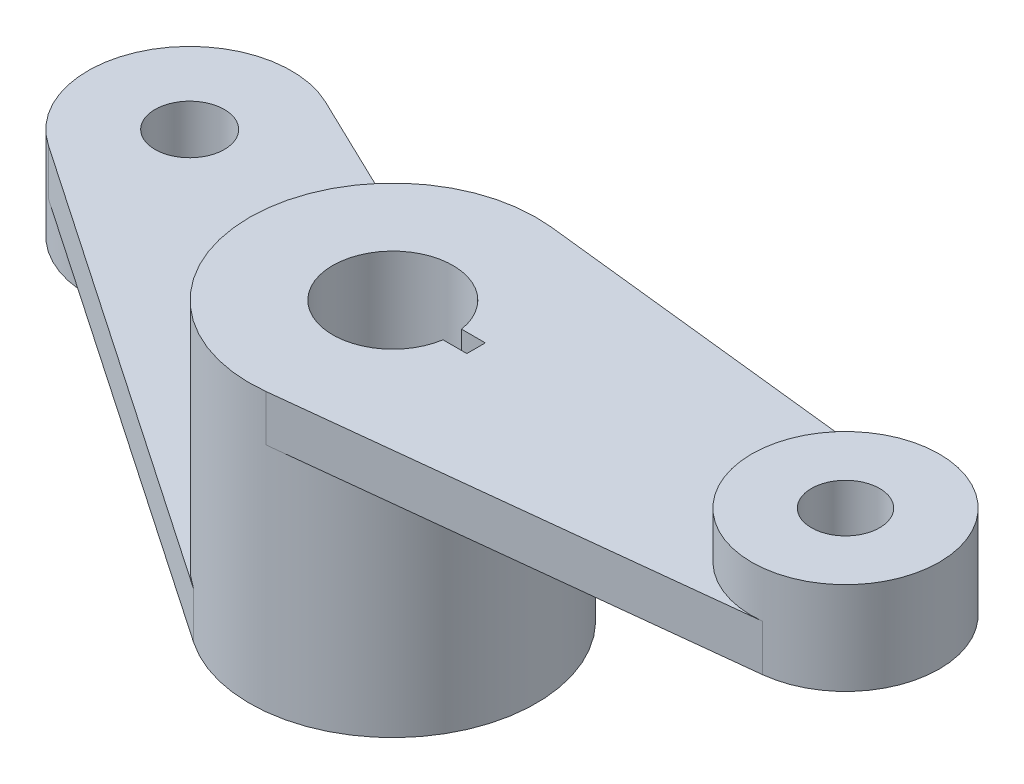
ISO-10303-21;
HEADER;
FILE_DESCRIPTION(('STEP AP214'),'2;1');
FILE_NAME('part.step','',(''),(''),'','','');
FILE_SCHEMA(('AUTOMOTIVE_DESIGN { 1 0 10303 214 1 1 1 1 }'));
ENDSEC;
DATA;
#1=APPLICATION_CONTEXT('core data for automotive mechanical design processes');
#2=APPLICATION_PROTOCOL_DEFINITION('international standard','automotive_design',2000,#1);
#3=PRODUCT_CONTEXT('',#1,'mechanical');
#4=PRODUCT('Part','Part','',(#3));
#5=PRODUCT_RELATED_PRODUCT_CATEGORY('part','',(#4));
#6=PRODUCT_DEFINITION_FORMATION('','',#4);
#7=PRODUCT_DEFINITION_CONTEXT('part definition',#1,'design');
#8=PRODUCT_DEFINITION('design','',#6,#7);
#9=PRODUCT_DEFINITION_SHAPE('','',#8);
#10=(LENGTH_UNIT() NAMED_UNIT(*) SI_UNIT(.MILLI.,.METRE.));
#11=(NAMED_UNIT(*) PLANE_ANGLE_UNIT() SI_UNIT($,.RADIAN.));
#12=(NAMED_UNIT(*) SI_UNIT($,.STERADIAN.) SOLID_ANGLE_UNIT());
#13=UNCERTAINTY_MEASURE_WITH_UNIT(LENGTH_MEASURE(1.E-05),#10,'distance_accuracy_value','');
#14=(GEOMETRIC_REPRESENTATION_CONTEXT(3) GLOBAL_UNCERTAINTY_ASSIGNED_CONTEXT((#13)) GLOBAL_UNIT_ASSIGNED_CONTEXT((#10,
#11,#12)) REPRESENTATION_CONTEXT('',''));
#15=CARTESIAN_POINT('',(0.,0.,0.));
#16=DIRECTION('',(0.,0.,1.));
#17=DIRECTION('',(1.,0.,0.));
#18=AXIS2_PLACEMENT_3D('',#15,#16,#17);
#19=CARTESIAN_POINT('',(0.,0.,0.));
#20=DIRECTION('',(0.,1.,0.));
#21=DIRECTION('',(0.,0.,1.));
#22=AXIS2_PLACEMENT_3D('',#19,#20,#21);
#23=PLANE('',#22);
#24=CARTESIAN_POINT('',(0.,0.,0.));
#25=DIRECTION('',(0.,1.,0.));
#26=DIRECTION('',(0.,0.,1.));
#27=AXIS2_PLACEMENT_3D('',#24,#25,#26);
#28=CIRCLE('',#27,31.);
#29=CARTESIAN_POINT('',(-17.4698538370627,0.,25.6086744465946));
#30=VERTEX_POINT('',#29);
#31=CARTESIAN_POINT('',(13.4428357094651,0.,-27.9336744465946));
#32=VERTEX_POINT('',#31);
#33=EDGE_CURVE('E44',#30,#32,#28,.T.);
#34=ORIENTED_EDGE('',*,*,#33,.F.);
#35=DIRECTION('',(0.826086272470793,0.,0.563543672163313));
#36=VECTOR('',#35,1.);
#37=CARTESIAN_POINT('',(-17.4698538370627,0.,25.6086744465946));
#38=LINE('',#37,#36);
#39=CARTESIAN_POINT('',(-116.321009241725,0.,-41.8261020056427));
#40=VERTEX_POINT('',#39);
#41=EDGE_CURVE('E155',#40,#30,#38,.T.);
#42=ORIENTED_EDGE('',*,*,#41,.F.);
#43=CARTESIAN_POINT('',(-103.923048454133,0.,-60.0000000000002));
#44=DIRECTION('',(0.,-1.,0.));
#45=DIRECTION('',(0.,0.,-1.));
#46=AXIS2_PLACEMENT_3D('',#43,#44,#45);
#47=CIRCLE('',#46,22.);
#48=CARTESIAN_POINT('',(-94.3829714990283,0.,-79.8238979943576));
#49=VERTEX_POINT('',#48);
#50=EDGE_CURVE('E162',#49,#40,#47,.T.);
#51=ORIENTED_EDGE('',*,*,#50,.F.);
#52=DIRECTION('',(0.901086272470793,0.,0.433639861595647));
#53=VECTOR('',#52,1.);
#54=CARTESIAN_POINT('',(13.4428357094651,0.,-27.9336744465946));
#55=LINE('',#54,#53);
#56=EDGE_CURVE('E150',#49,#32,#55,.T.);
#57=ORIENTED_EDGE('',*,*,#56,.T.);
#58=EDGE_LOOP('',(#34,#42,#51,#57));
#59=FACE_BOUND('',#58,.T.);
#60=DIRECTION('',(0.,0.,-1.));
#61=VECTOR('',#60,1.);
#62=CARTESIAN_POINT('',(18.,0.,2.));
#63=LINE('',#62,#61);
#64=CARTESIAN_POINT('',(18.,0.,2.));
#65=VERTEX_POINT('',#64);
#66=CARTESIAN_POINT('',(18.,0.,-2.));
#67=VERTEX_POINT('',#66);
#68=EDGE_CURVE('E216',#65,#67,#63,.T.);
#69=ORIENTED_EDGE('',*,*,#68,.T.);
#70=DIRECTION('',(-1.,0.,0.));
#71=VECTOR('',#70,1.);
#72=CARTESIAN_POINT('',(12.8452325786651,0.,-2.));
#73=LINE('',#72,#71);
#74=CARTESIAN_POINT('',(12.8452325786651,0.,-2.));
#75=VERTEX_POINT('',#74);
#76=EDGE_CURVE('E225',#67,#75,#73,.T.);
#77=ORIENTED_EDGE('',*,*,#76,.T.);
#78=CARTESIAN_POINT('',(0.,0.,0.));
#79=DIRECTION('',(0.,1.,0.));
#80=DIRECTION('',(0.,0.,1.));
#81=AXIS2_PLACEMENT_3D('',#78,#79,#80);
#82=CIRCLE('',#81,13.);
#83=CARTESIAN_POINT('',(12.8452325786651,0.,2.));
#84=VERTEX_POINT('',#83);
#85=EDGE_CURVE('E223',#75,#84,#82,.T.);
#86=ORIENTED_EDGE('',*,*,#85,.T.);
#87=DIRECTION('',(1.,0.,0.));
#88=VECTOR('',#87,1.);
#89=CARTESIAN_POINT('',(12.8452325786651,0.,2.));
#90=LINE('',#89,#88);
#91=EDGE_CURVE('E226',#84,#65,#90,.T.);
#92=ORIENTED_EDGE('',*,*,#91,.T.);
#93=EDGE_LOOP('',(#69,#77,#86,#92));
#94=FACE_BOUND('',#93,.T.);
#95=ADVANCED_FACE('F41',(#59,#94),#23,.F.);
#96=CARTESIAN_POINT('',(0.,50.,0.));
#97=DIRECTION('',(0.,-1.,0.));
#98=DIRECTION('',(0.,0.,-1.));
#99=AXIS2_PLACEMENT_3D('',#96,#97,#98);
#100=CYLINDRICAL_SURFACE('',#99,31.);
#101=CARTESIAN_POINT('',(0.,10.,0.));
#102=DIRECTION('',(0.,-1.,0.));
#103=DIRECTION('',(0.,0.,-1.));
#104=AXIS2_PLACEMENT_3D('',#101,#102,#103);
#105=CIRCLE('',#104,31.);
#106=CARTESIAN_POINT('',(-17.4698538370627,10.,25.6086744465946));
#107=VERTEX_POINT('',#106);
#108=CARTESIAN_POINT('',(13.4428357094651,10.,-27.9336744465946));
#109=VERTEX_POINT('',#108);
#110=EDGE_CURVE('E58',#107,#109,#105,.T.);
#111=ORIENTED_EDGE('',*,*,#110,.F.);
#112=DIRECTION('',(0.,-1.,0.));
#113=VECTOR('',#112,1.);
#114=CARTESIAN_POINT('',(-17.4698538370627,10.,25.6086744465946));
#115=LINE('',#114,#113);
#116=EDGE_CURVE('E170',#107,#30,#115,.T.);
#117=ORIENTED_EDGE('',*,*,#116,.T.);
#118=ORIENTED_EDGE('',*,*,#33,.T.);
#119=DIRECTION('',(0.,-1.,0.));
#120=VECTOR('',#119,1.);
#121=CARTESIAN_POINT('',(13.4428357094651,10.,-27.9336744465946));
#122=LINE('',#121,#120);
#123=EDGE_CURVE('E57',#109,#32,#122,.T.);
#124=ORIENTED_EDGE('',*,*,#123,.F.);
#125=EDGE_LOOP('',(#111,#117,#118,#124));
#126=FACE_BOUND('',#125,.T.);
#127=CARTESIAN_POINT('',(0.,50.,0.));
#128=DIRECTION('',(0.,1.,0.));
#129=DIRECTION('',(0.,0.,1.));
#130=AXIS2_PLACEMENT_3D('',#127,#128,#129);
#131=CIRCLE('',#130,31.);
#132=CARTESIAN_POINT('',(3.39474140315786,50.,30.8135640717799));
#133=VERTEX_POINT('',#132);
#134=CARTESIAN_POINT('',(3.39474140315786,50.,-30.8135640717799));
#135=VERTEX_POINT('',#134);
#136=EDGE_CURVE('E11',#133,#135,#131,.T.);
#137=ORIENTED_EDGE('',*,*,#136,.F.);
#138=DIRECTION('',(0.,-1.,0.));
#139=VECTOR('',#138,1.);
#140=CARTESIAN_POINT('',(3.39474140315786,60.,30.8135640717799));
#141=LINE('',#140,#139);
#142=CARTESIAN_POINT('',(3.39474140315786,60.,30.8135640717799));
#143=VERTEX_POINT('',#142);
#144=EDGE_CURVE('E214',#143,#133,#141,.T.);
#145=ORIENTED_EDGE('',*,*,#144,.F.);
#146=CARTESIAN_POINT('',(0.,60.,0.));
#147=DIRECTION('',(0.,1.,0.));
#148=DIRECTION('',(0.,0.,1.));
#149=AXIS2_PLACEMENT_3D('',#146,#147,#148);
#150=CIRCLE('',#149,31.);
#151=CARTESIAN_POINT('',(3.39474140315786,60.,-30.8135640717799));
#152=VERTEX_POINT('',#151);
#153=EDGE_CURVE('E183',#152,#143,#150,.T.);
#154=ORIENTED_EDGE('',*,*,#153,.F.);
#155=DIRECTION('',(0.,-1.,0.));
#156=VECTOR('',#155,1.);
#157=CARTESIAN_POINT('',(3.39474140315786,60.,-30.8135640717799));
#158=LINE('',#157,#156);
#159=EDGE_CURVE('E217',#152,#135,#158,.T.);
#160=ORIENTED_EDGE('',*,*,#159,.T.);
#161=EDGE_LOOP('',(#137,#145,#154,#160));
#162=FACE_BOUND('',#161,.T.);
#163=ADVANCED_FACE('F43',(#126,#162),#100,.T.);
#164=CARTESIAN_POINT('',(18.,50.,2.));
#165=DIRECTION('',(-1.,0.,0.));
#166=DIRECTION('',(0.,0.,1.));
#167=AXIS2_PLACEMENT_3D('',#164,#165,#166);
#168=PLANE('',#167);
#169=ORIENTED_EDGE('',*,*,#68,.F.);
#170=DIRECTION('',(0.,-1.,0.));
#171=VECTOR('',#170,1.);
#172=CARTESIAN_POINT('',(18.,50.,2.));
#173=LINE('',#172,#171);
#174=CARTESIAN_POINT('',(18.,60.,2.));
#175=VERTEX_POINT('',#174);
#176=EDGE_CURVE('E233',#175,#65,#173,.T.);
#177=ORIENTED_EDGE('',*,*,#176,.F.);
#178=DIRECTION('',(0.,0.,1.));
#179=VECTOR('',#178,1.);
#180=CARTESIAN_POINT('',(18.,60.,0.));
#181=LINE('',#180,#179);
#182=CARTESIAN_POINT('',(18.,60.,-2.));
#183=VERTEX_POINT('',#182);
#184=EDGE_CURVE('E196',#183,#175,#181,.T.);
#185=ORIENTED_EDGE('',*,*,#184,.F.);
#186=DIRECTION('',(0.,-1.,0.));
#187=VECTOR('',#186,1.);
#188=CARTESIAN_POINT('',(18.,50.,-2.));
#189=LINE('',#188,#187);
#190=EDGE_CURVE('E238',#183,#67,#189,.T.);
#191=ORIENTED_EDGE('',*,*,#190,.T.);
#192=EDGE_LOOP('',(#169,#177,#185,#191));
#193=FACE_BOUND('',#192,.T.);
#194=ADVANCED_FACE('F263',(#193),#168,.T.);
#195=CARTESIAN_POINT('',(12.8452325786651,50.,-2.));
#196=DIRECTION('',(0.,0.,1.));
#197=DIRECTION('',(1.,0.,0.));
#198=AXIS2_PLACEMENT_3D('',#195,#196,#197);
#199=PLANE('',#198);
#200=ORIENTED_EDGE('',*,*,#76,.F.);
#201=ORIENTED_EDGE('',*,*,#190,.F.);
#202=DIRECTION('',(1.,0.,0.));
#203=VECTOR('',#202,1.);
#204=CARTESIAN_POINT('',(0.,60.,-2.));
#205=LINE('',#204,#203);
#206=CARTESIAN_POINT('',(12.8452325786651,60.,-2.));
#207=VERTEX_POINT('',#206);
#208=EDGE_CURVE('E197',#207,#183,#205,.T.);
#209=ORIENTED_EDGE('',*,*,#208,.F.);
#210=DIRECTION('',(0.,-1.,0.));
#211=VECTOR('',#210,1.);
#212=CARTESIAN_POINT('',(12.8452325786651,50.,-2.));
#213=LINE('',#212,#211);
#214=EDGE_CURVE('E236',#207,#75,#213,.T.);
#215=ORIENTED_EDGE('',*,*,#214,.T.);
#216=EDGE_LOOP('',(#200,#201,#209,#215));
#217=FACE_BOUND('',#216,.T.);
#218=ADVANCED_FACE('F266',(#217),#199,.T.);
#219=CARTESIAN_POINT('',(0.,50.,0.));
#220=DIRECTION('',(0.,-1.,0.));
#221=DIRECTION('',(0.,0.,-1.));
#222=AXIS2_PLACEMENT_3D('',#219,#220,#221);
#223=CYLINDRICAL_SURFACE('',#222,13.);
#224=ORIENTED_EDGE('',*,*,#85,.F.);
#225=ORIENTED_EDGE('',*,*,#214,.F.);
#226=CARTESIAN_POINT('',(0.,60.,0.));
#227=DIRECTION('',(0.,1.,0.));
#228=DIRECTION('',(0.,0.,1.));
#229=AXIS2_PLACEMENT_3D('',#226,#227,#228);
#230=CIRCLE('',#229,13.);
#231=CARTESIAN_POINT('',(12.8452325786651,60.,2.));
#232=VERTEX_POINT('',#231);
#233=EDGE_CURVE('E194',#232,#207,#230,.F.);
#234=ORIENTED_EDGE('',*,*,#233,.F.);
#235=DIRECTION('',(0.,-1.,0.));
#236=VECTOR('',#235,1.);
#237=CARTESIAN_POINT('',(12.8452325786651,50.,2.));
#238=LINE('',#237,#236);
#239=EDGE_CURVE('E234',#232,#84,#238,.T.);
#240=ORIENTED_EDGE('',*,*,#239,.T.);
#241=EDGE_LOOP('',(#224,#225,#234,#240));
#242=FACE_BOUND('',#241,.T.);
#243=ADVANCED_FACE('F275',(#242),#223,.F.);
#244=CARTESIAN_POINT('',(12.8452325786651,50.,2.));
#245=DIRECTION('',(0.,0.,-1.));
#246=DIRECTION('',(-1.,0.,0.));
#247=AXIS2_PLACEMENT_3D('',#244,#245,#246);
#248=PLANE('',#247);
#249=ORIENTED_EDGE('',*,*,#91,.F.);
#250=ORIENTED_EDGE('',*,*,#239,.F.);
#251=DIRECTION('',(-1.,0.,0.));
#252=VECTOR('',#251,1.);
#253=CARTESIAN_POINT('',(0.,60.,2.));
#254=LINE('',#253,#252);
#255=EDGE_CURVE('E205',#175,#232,#254,.T.);
#256=ORIENTED_EDGE('',*,*,#255,.F.);
#257=ORIENTED_EDGE('',*,*,#176,.T.);
#258=EDGE_LOOP('',(#249,#250,#256,#257));
#259=FACE_BOUND('',#258,.T.);
#260=ADVANCED_FACE('F277',(#259),#248,.T.);
#261=CARTESIAN_POINT('',(0.,50.,0.));
#262=DIRECTION('',(0.,1.,0.));
#263=DIRECTION('',(0.,0.,1.));
#264=AXIS2_PLACEMENT_3D('',#261,#262,#263);
#265=PLANE('',#264);
#266=DIRECTION('',(0.993985937799352,0.,-0.109507787198641));
#267=VECTOR('',#266,1.);
#268=CARTESIAN_POINT('',(3.39474140315786,50.,30.8135640717799));
#269=LINE('',#268,#267);
#270=CARTESIAN_POINT('',(100.096839243233,50.,20.1598592765409));
#271=VERTEX_POINT('',#270);
#272=EDGE_CURVE('E184',#133,#271,#269,.T.);
#273=ORIENTED_EDGE('',*,*,#272,.F.);
#274=ORIENTED_EDGE('',*,*,#136,.T.);
#275=DIRECTION('',(0.993985937799352,0.,0.109507787198641));
#276=VECTOR('',#275,1.);
#277=CARTESIAN_POINT('',(3.39474140315786,50.,-30.8135640717799));
#278=LINE('',#277,#276);
#279=CARTESIAN_POINT('',(100.096839243233,50.,-20.1598592765409));
#280=VERTEX_POINT('',#279);
#281=EDGE_CURVE('E180',#135,#280,#278,.T.);
#282=ORIENTED_EDGE('',*,*,#281,.T.);
#283=CARTESIAN_POINT('',(97.8758203176558,50.,0.));
#284=DIRECTION('',(0.,1.,0.));
#285=DIRECTION('',(0.,0.,1.));
#286=AXIS2_PLACEMENT_3D('',#283,#284,#285);
#287=CIRCLE('',#286,20.2818354967618);
#288=EDGE_CURVE('E172',#271,#280,#287,.T.);
#289=ORIENTED_EDGE('',*,*,#288,.F.);
#290=EDGE_LOOP('',(#273,#274,#282,#289));
#291=FACE_BOUND('',#290,.T.);
#292=CARTESIAN_POINT('',(97.8758203176558,50.,0.));
#293=DIRECTION('',(0.,1.,0.));
#294=DIRECTION('',(0.,0.,1.));
#295=AXIS2_PLACEMENT_3D('',#292,#293,#294);
#296=CIRCLE('',#295,7.37420564037151);
#297=CARTESIAN_POINT('',(97.8758203176558,50.,7.37420564037151));
#298=VERTEX_POINT('',#297);
#299=EDGE_CURVE('E168',#298,#298,#296,.T.);
#300=ORIENTED_EDGE('',*,*,#299,.T.);
#301=EDGE_LOOP('',(#300));
#302=FACE_BOUND('',#301,.T.);
#303=ADVANCED_FACE('F278',(#291,#302),#265,.F.);
#304=CARTESIAN_POINT('',(3.39474140315786,60.,-30.8135640717799));
#305=DIRECTION('',(0.109507787198641,0.,-0.993985937799352));
#306=DIRECTION('',(-0.993985937799352,0.,-0.109507787198641));
#307=AXIS2_PLACEMENT_3D('',#304,#305,#306);
#308=PLANE('',#307);
#309=ORIENTED_EDGE('',*,*,#281,.F.);
#310=ORIENTED_EDGE('',*,*,#159,.F.);
#311=DIRECTION('',(0.993985937799352,0.,0.109507787198641));
#312=VECTOR('',#311,1.);
#313=CARTESIAN_POINT('',(3.39474140315786,60.,-30.8135640717799));
#314=LINE('',#313,#312);
#315=CARTESIAN_POINT('',(100.096839243233,60.,-20.1598592765409));
#316=VERTEX_POINT('',#315);
#317=EDGE_CURVE('E185',#152,#316,#314,.T.);
#318=ORIENTED_EDGE('',*,*,#317,.T.);
#319=DIRECTION('',(0.,-1.,0.));
#320=VECTOR('',#319,1.);
#321=CARTESIAN_POINT('',(100.096839243233,60.,-20.1598592765409));
#322=LINE('',#321,#320);
#323=EDGE_CURVE('E203',#316,#280,#322,.T.);
#324=ORIENTED_EDGE('',*,*,#323,.T.);
#325=EDGE_LOOP('',(#309,#310,#318,#324));
#326=FACE_BOUND('',#325,.T.);
#327=ADVANCED_FACE('F285',(#326),#308,.T.);
#328=CARTESIAN_POINT('',(3.39474140315786,60.,30.8135640717799));
#329=DIRECTION('',(-0.109507787198641,0.,-0.993985937799352));
#330=DIRECTION('',(-0.993985937799352,0.,0.109507787198641));
#331=AXIS2_PLACEMENT_3D('',#328,#329,#330);
#332=PLANE('',#331);
#333=ORIENTED_EDGE('',*,*,#272,.T.);
#334=DIRECTION('',(0.,-1.,0.));
#335=VECTOR('',#334,1.);
#336=CARTESIAN_POINT('',(100.096839243233,60.,20.1598592765409));
#337=LINE('',#336,#335);
#338=CARTESIAN_POINT('',(100.096839243233,60.,20.1598592765409));
#339=VERTEX_POINT('',#338);
#340=EDGE_CURVE('E208',#339,#271,#337,.T.);
#341=ORIENTED_EDGE('',*,*,#340,.F.);
#342=DIRECTION('',(0.993985937799352,0.,-0.109507787198641));
#343=VECTOR('',#342,1.);
#344=CARTESIAN_POINT('',(3.39474140315786,60.,30.8135640717799));
#345=LINE('',#344,#343);
#346=EDGE_CURVE('E190',#143,#339,#345,.T.);
#347=ORIENTED_EDGE('',*,*,#346,.F.);
#348=ORIENTED_EDGE('',*,*,#144,.T.);
#349=EDGE_LOOP('',(#333,#341,#347,#348));
#350=FACE_BOUND('',#349,.T.);
#351=ADVANCED_FACE('F283',(#350),#332,.F.);
#352=CARTESIAN_POINT('',(0.,60.,0.));
#353=DIRECTION('',(0.,1.,0.));
#354=DIRECTION('',(0.,0.,1.));
#355=AXIS2_PLACEMENT_3D('',#352,#353,#354);
#356=PLANE('',#355);
#357=ORIENTED_EDGE('',*,*,#317,.F.);
#358=ORIENTED_EDGE('',*,*,#153,.T.);
#359=ORIENTED_EDGE('',*,*,#346,.T.);
#360=CARTESIAN_POINT('',(97.8758203176558,60.,0.));
#361=DIRECTION('',(0.,1.,0.));
#362=DIRECTION('',(0.,0.,1.));
#363=AXIS2_PLACEMENT_3D('',#360,#361,#362);
#364=CIRCLE('',#363,20.2818354967618);
#365=EDGE_CURVE('E188',#316,#339,#364,.T.);
#366=ORIENTED_EDGE('',*,*,#365,.F.);
#367=EDGE_LOOP('',(#357,#358,#359,#366));
#368=FACE_BOUND('',#367,.T.);
#369=ORIENTED_EDGE('',*,*,#233,.T.);
#370=ORIENTED_EDGE('',*,*,#208,.T.);
#371=ORIENTED_EDGE('',*,*,#184,.T.);
#372=ORIENTED_EDGE('',*,*,#255,.T.);
#373=EDGE_LOOP('',(#369,#370,#371,#372));
#374=FACE_BOUND('',#373,.T.);
#375=ADVANCED_FACE('F286',(#368,#374),#356,.T.);
#376=CARTESIAN_POINT('',(97.8758203176558,70.,0.));
#377=DIRECTION('',(0.,-1.,0.));
#378=DIRECTION('',(0.,0.,-1.));
#379=AXIS2_PLACEMENT_3D('',#376,#377,#378);
#380=CYLINDRICAL_SURFACE('',#379,20.2818354967618);
#381=CARTESIAN_POINT('',(97.8758203176558,70.,0.));
#382=DIRECTION('',(0.,1.,0.));
#383=DIRECTION('',(0.,0.,1.));
#384=AXIS2_PLACEMENT_3D('',#381,#382,#383);
#385=CIRCLE('',#384,20.2818354967618);
#386=CARTESIAN_POINT('',(97.8758203176558,70.,20.2818354967618));
#387=VERTEX_POINT('',#386);
#388=EDGE_CURVE('E173',#387,#387,#385,.T.);
#389=ORIENTED_EDGE('',*,*,#388,.F.);
#390=EDGE_LOOP('',(#389));
#391=FACE_BOUND('',#390,.T.);
#392=ORIENTED_EDGE('',*,*,#288,.T.);
#393=ORIENTED_EDGE('',*,*,#323,.F.);
#394=ORIENTED_EDGE('',*,*,#365,.T.);
#395=ORIENTED_EDGE('',*,*,#340,.T.);
#396=EDGE_LOOP('',(#392,#393,#394,#395));
#397=FACE_BOUND('',#396,.T.);
#398=ADVANCED_FACE('F298',(#391,#397),#380,.T.);
#399=CARTESIAN_POINT('',(97.8758203176558,70.,0.));
#400=DIRECTION('',(0.,-1.,0.));
#401=DIRECTION('',(0.,0.,-1.));
#402=AXIS2_PLACEMENT_3D('',#399,#400,#401);
#403=CYLINDRICAL_SURFACE('',#402,7.37420564037151);
#404=CARTESIAN_POINT('',(97.8758203176558,70.,0.));
#405=DIRECTION('',(0.,1.,0.));
#406=DIRECTION('',(0.,0.,1.));
#407=AXIS2_PLACEMENT_3D('',#404,#405,#406);
#408=CIRCLE('',#407,7.37420564037151);
#409=CARTESIAN_POINT('',(97.8758203176558,70.,7.37420564037151));
#410=VERTEX_POINT('',#409);
#411=EDGE_CURVE('E167',#410,#410,#408,.T.);
#412=ORIENTED_EDGE('',*,*,#411,.T.);
#413=EDGE_LOOP('',(#412));
#414=FACE_BOUND('',#413,.T.);
#415=ORIENTED_EDGE('',*,*,#299,.F.);
#416=EDGE_LOOP('',(#415));
#417=FACE_BOUND('',#416,.T.);
#418=ADVANCED_FACE('F259',(#414,#417),#403,.F.);
#419=CARTESIAN_POINT('',(0.,70.,0.));
#420=DIRECTION('',(0.,1.,0.));
#421=DIRECTION('',(0.,0.,1.));
#422=AXIS2_PLACEMENT_3D('',#419,#420,#421);
#423=PLANE('',#422);
#424=ORIENTED_EDGE('',*,*,#411,.F.);
#425=EDGE_LOOP('',(#424));
#426=FACE_BOUND('',#425,.T.);
#427=ORIENTED_EDGE('',*,*,#388,.T.);
#428=EDGE_LOOP('',(#427));
#429=FACE_BOUND('',#428,.T.);
#430=ADVANCED_FACE('F249',(#426,#429),#423,.T.);
#431=CARTESIAN_POINT('',(-17.4698538370627,10.,25.6086744465946));
#432=DIRECTION('',(0.563543672163313,0.,-0.826086272470793));
#433=DIRECTION('',(-0.826086272470793,0.,-0.563543672163313));
#434=AXIS2_PLACEMENT_3D('',#431,#432,#433);
#435=PLANE('',#434);
#436=ORIENTED_EDGE('',*,*,#41,.T.);
#437=ORIENTED_EDGE('',*,*,#116,.F.);
#438=DIRECTION('',(0.826086272470793,0.,0.563543672163313));
#439=VECTOR('',#438,1.);
#440=CARTESIAN_POINT('',(-17.4698538370627,10.,25.6086744465946));
#441=LINE('',#440,#439);
#442=CARTESIAN_POINT('',(-116.321009241725,10.,-41.8261020056427));
#443=VERTEX_POINT('',#442);
#444=EDGE_CURVE('E149',#443,#107,#441,.T.);
#445=ORIENTED_EDGE('',*,*,#444,.F.);
#446=DIRECTION('',(0.,-1.,0.));
#447=VECTOR('',#446,1.);
#448=CARTESIAN_POINT('',(-116.321009241725,10.,-41.8261020056427));
#449=LINE('',#448,#447);
#450=EDGE_CURVE('E131',#443,#40,#449,.T.);
#451=ORIENTED_EDGE('',*,*,#450,.T.);
#452=EDGE_LOOP('',(#436,#437,#445,#451));
#453=FACE_BOUND('',#452,.T.);
#454=ADVANCED_FACE('F247',(#453),#435,.F.);
#455=CARTESIAN_POINT('',(13.4428357094651,10.,-27.9336744465946));
#456=DIRECTION('',(0.433639861595647,0.,-0.901086272470793));
#457=DIRECTION('',(-0.901086272470793,0.,-0.433639861595647));
#458=AXIS2_PLACEMENT_3D('',#455,#456,#457);
#459=PLANE('',#458);
#460=ORIENTED_EDGE('',*,*,#56,.F.);
#461=DIRECTION('',(0.,-1.,0.));
#462=VECTOR('',#461,1.);
#463=CARTESIAN_POINT('',(-94.3829714990283,10.,-79.8238979943576));
#464=LINE('',#463,#462);
#465=CARTESIAN_POINT('',(-94.3829714990283,10.,-79.8238979943576));
#466=VERTEX_POINT('',#465);
#467=EDGE_CURVE('E132',#466,#49,#464,.T.);
#468=ORIENTED_EDGE('',*,*,#467,.F.);
#469=DIRECTION('',(0.901086272470793,0.,0.433639861595647));
#470=VECTOR('',#469,1.);
#471=CARTESIAN_POINT('',(13.4428357094651,10.,-27.9336744465946));
#472=LINE('',#471,#470);
#473=EDGE_CURVE('E143',#466,#109,#472,.T.);
#474=ORIENTED_EDGE('',*,*,#473,.T.);
#475=ORIENTED_EDGE('',*,*,#123,.T.);
#476=EDGE_LOOP('',(#460,#468,#474,#475));
#477=FACE_BOUND('',#476,.T.);
#478=ADVANCED_FACE('F144',(#477),#459,.T.);
#479=CARTESIAN_POINT('',(0.,10.,0.));
#480=DIRECTION('',(0.,-1.,0.));
#481=DIRECTION('',(0.,0.,-1.));
#482=AXIS2_PLACEMENT_3D('',#479,#480,#481);
#483=PLANE('',#482);
#484=ORIENTED_EDGE('',*,*,#473,.F.);
#485=CARTESIAN_POINT('',(-103.923048454133,10.,-60.0000000000002));
#486=DIRECTION('',(0.,-1.,0.));
#487=DIRECTION('',(0.,0.,-1.));
#488=AXIS2_PLACEMENT_3D('',#485,#486,#487);
#489=CIRCLE('',#488,22.);
#490=EDGE_CURVE('E130',#443,#466,#489,.T.);
#491=ORIENTED_EDGE('',*,*,#490,.F.);
#492=ORIENTED_EDGE('',*,*,#444,.T.);
#493=ORIENTED_EDGE('',*,*,#110,.T.);
#494=EDGE_LOOP('',(#484,#491,#492,#493));
#495=FACE_BOUND('',#494,.T.);
#496=CARTESIAN_POINT('',(-103.923048454133,10.,-60.0000000000002));
#497=DIRECTION('',(0.,-1.,0.));
#498=DIRECTION('',(0.,0.,-1.));
#499=AXIS2_PLACEMENT_3D('',#496,#497,#498);
#500=CIRCLE('',#499,7.50000000000001);
#501=CARTESIAN_POINT('',(-103.923048454133,10.,-67.5000000000002));
#502=VERTEX_POINT('',#501);
#503=EDGE_CURVE('E136',#502,#502,#500,.T.);
#504=ORIENTED_EDGE('',*,*,#503,.T.);
#505=EDGE_LOOP('',(#504));
#506=FACE_BOUND('',#505,.T.);
#507=ADVANCED_FACE('F148',(#495,#506),#483,.F.);
#508=CARTESIAN_POINT('',(-103.923048454133,-10.,-60.0000000000002));
#509=DIRECTION('',(0.,1.,0.));
#510=DIRECTION('',(0.,0.,1.));
#511=AXIS2_PLACEMENT_3D('',#508,#509,#510);
#512=CYLINDRICAL_SURFACE('',#511,7.50000000000001);
#513=CARTESIAN_POINT('',(-103.923048454133,-10.,-60.0000000000002));
#514=DIRECTION('',(0.,-1.,0.));
#515=DIRECTION('',(0.,0.,-1.));
#516=AXIS2_PLACEMENT_3D('',#513,#514,#515);
#517=CIRCLE('',#516,7.50000000000001);
#518=CARTESIAN_POINT('',(-103.923048454133,-10.,-67.5000000000002));
#519=VERTEX_POINT('',#518);
#520=EDGE_CURVE('E139',#519,#519,#517,.T.);
#521=ORIENTED_EDGE('',*,*,#520,.T.);
#522=EDGE_LOOP('',(#521));
#523=FACE_BOUND('',#522,.T.);
#524=ORIENTED_EDGE('',*,*,#503,.F.);
#525=EDGE_LOOP('',(#524));
#526=FACE_BOUND('',#525,.T.);
#527=ADVANCED_FACE('F432',(#523,#526),#512,.F.);
#528=CARTESIAN_POINT('',(-103.923048454133,-10.,-60.0000000000002));
#529=DIRECTION('',(0.,1.,0.));
#530=DIRECTION('',(0.,0.,1.));
#531=AXIS2_PLACEMENT_3D('',#528,#529,#530);
#532=CYLINDRICAL_SURFACE('',#531,22.);
#533=ORIENTED_EDGE('',*,*,#450,.F.);
#534=ORIENTED_EDGE('',*,*,#490,.T.);
#535=ORIENTED_EDGE('',*,*,#467,.T.);
#536=ORIENTED_EDGE('',*,*,#50,.T.);
#537=EDGE_LOOP('',(#533,#534,#535,#536));
#538=FACE_BOUND('',#537,.T.);
#539=CARTESIAN_POINT('',(-103.923048454133,-10.,-60.0000000000002));
#540=DIRECTION('',(0.,-1.,0.));
#541=DIRECTION('',(0.,0.,-1.));
#542=AXIS2_PLACEMENT_3D('',#539,#540,#541);
#543=CIRCLE('',#542,22.);
#544=CARTESIAN_POINT('',(-103.923048454133,-10.,-82.0000000000001));
#545=VERTEX_POINT('',#544);
#546=EDGE_CURVE('E159',#545,#545,#543,.T.);
#547=ORIENTED_EDGE('',*,*,#546,.F.);
#548=EDGE_LOOP('',(#547));
#549=FACE_BOUND('',#548,.T.);
#550=ADVANCED_FACE('F126',(#538,#549),#532,.T.);
#551=CARTESIAN_POINT('',(0.,-10.,0.));
#552=DIRECTION('',(0.,-1.,0.));
#553=DIRECTION('',(0.,0.,-1.));
#554=AXIS2_PLACEMENT_3D('',#551,#552,#553);
#555=PLANE('',#554);
#556=ORIENTED_EDGE('',*,*,#520,.F.);
#557=EDGE_LOOP('',(#556));
#558=FACE_BOUND('',#557,.T.);
#559=ORIENTED_EDGE('',*,*,#546,.T.);
#560=EDGE_LOOP('',(#559));
#561=FACE_BOUND('',#560,.T.);
#562=ADVANCED_FACE('F448',(#558,#561),#555,.T.);
#563=CLOSED_SHELL('',(#95,#163,#194,#218,#243,#260,#303,#327,#351,#375,#398,#418,#430,#454,#478,
#507,#527,#550,#562));
#564=MANIFOLD_SOLID_BREP('B2',#563);
#565=ADVANCED_BREP_SHAPE_REPRESENTATION('',(#18,#564),#14);
#566=SHAPE_DEFINITION_REPRESENTATION(#9,#565);
ENDSEC;
END-ISO-10303-21;
